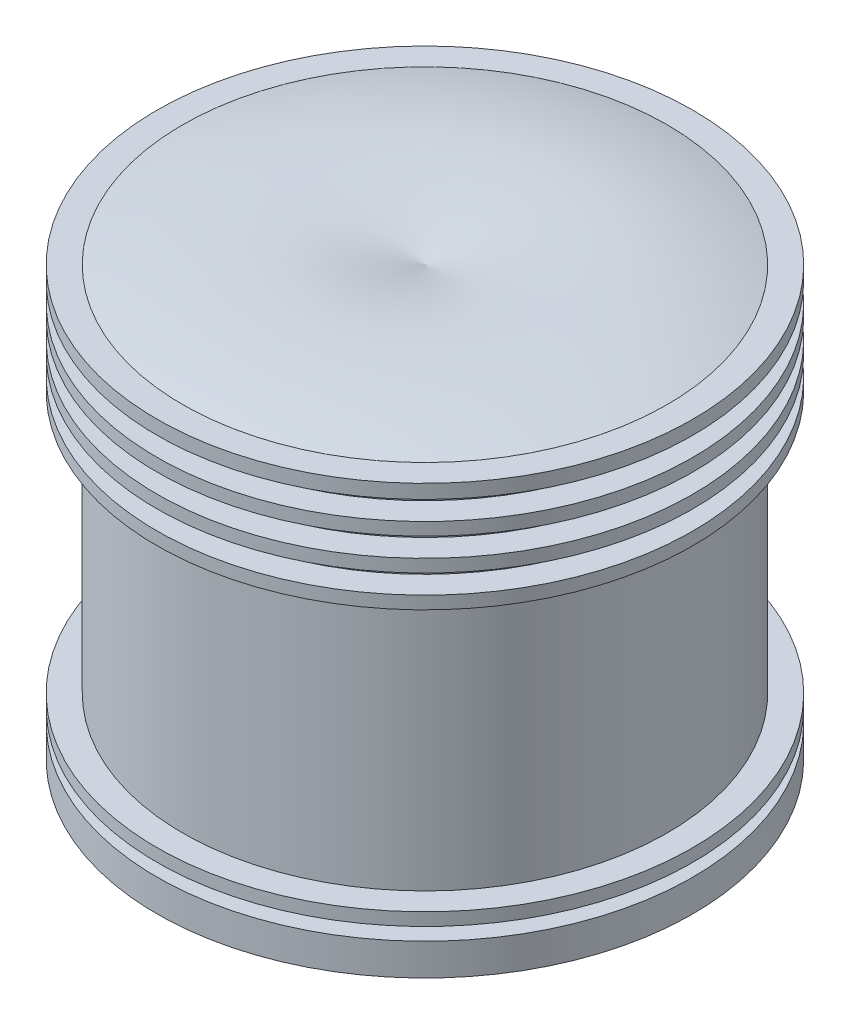
ISO-10303-21;
HEADER;
FILE_DESCRIPTION(('STEP AP214'),'2;1');
FILE_NAME('part.step','',(''),(''),'','','');
FILE_SCHEMA(('AUTOMOTIVE_DESIGN { 1 0 10303 214 1 1 1 1 }'));
ENDSEC;
DATA;
#1=APPLICATION_CONTEXT('core data for automotive mechanical design processes');
#2=APPLICATION_PROTOCOL_DEFINITION('international standard','automotive_design',2000,#1);
#3=PRODUCT_CONTEXT('',#1,'mechanical');
#4=PRODUCT('Part','Part','',(#3));
#5=PRODUCT_RELATED_PRODUCT_CATEGORY('part','',(#4));
#6=PRODUCT_DEFINITION_FORMATION('','',#4);
#7=PRODUCT_DEFINITION_CONTEXT('part definition',#1,'design');
#8=PRODUCT_DEFINITION('design','',#6,#7);
#9=PRODUCT_DEFINITION_SHAPE('','',#8);
#10=(LENGTH_UNIT() NAMED_UNIT(*) SI_UNIT(.MILLI.,.METRE.));
#11=(NAMED_UNIT(*) PLANE_ANGLE_UNIT() SI_UNIT($,.RADIAN.));
#12=(NAMED_UNIT(*) SI_UNIT($,.STERADIAN.) SOLID_ANGLE_UNIT());
#13=UNCERTAINTY_MEASURE_WITH_UNIT(LENGTH_MEASURE(1.E-05),#10,'distance_accuracy_value','');
#14=(GEOMETRIC_REPRESENTATION_CONTEXT(3) GLOBAL_UNCERTAINTY_ASSIGNED_CONTEXT((#13)) GLOBAL_UNIT_ASSIGNED_CONTEXT((#10,
#11,#12)) REPRESENTATION_CONTEXT('',''));
#15=CARTESIAN_POINT('',(0.,0.,0.));
#16=DIRECTION('',(0.,0.,1.));
#17=DIRECTION('',(1.,0.,0.));
#18=AXIS2_PLACEMENT_3D('',#15,#16,#17);
#19=CARTESIAN_POINT('',(0.,0.,0.));
#20=DIRECTION('',(0.,-1.,0.));
#21=DIRECTION('',(0.,0.,-1.));
#22=AXIS2_PLACEMENT_3D('',#19,#20,#21);
#23=CYLINDRICAL_SURFACE('',#22,42.);
#24=CARTESIAN_POINT('',(0.,9.,0.));
#25=DIRECTION('',(0.,-1.,0.));
#26=DIRECTION('',(0.,0.,-1.));
#27=AXIS2_PLACEMENT_3D('',#24,#25,#26);
#28=CIRCLE('',#27,42.);
#29=CARTESIAN_POINT('',(0.,9.,-42.));
#30=VERTEX_POINT('',#29);
#31=EDGE_CURVE('E171',#30,#30,#28,.T.);
#32=ORIENTED_EDGE('',*,*,#31,.T.);
#33=EDGE_LOOP('',(#32));
#34=FACE_BOUND('',#33,.T.);
#35=CARTESIAN_POINT('',(0.,7.,0.));
#36=DIRECTION('',(0.,-1.,0.));
#37=DIRECTION('',(0.,0.,-1.));
#38=AXIS2_PLACEMENT_3D('',#35,#36,#37);
#39=CIRCLE('',#38,42.);
#40=CARTESIAN_POINT('',(0.,7.,-42.));
#41=VERTEX_POINT('',#40);
#42=EDGE_CURVE('E11',#41,#41,#39,.T.);
#43=ORIENTED_EDGE('',*,*,#42,.F.);
#44=EDGE_LOOP('',(#43));
#45=FACE_BOUND('',#44,.T.);
#46=ADVANCED_FACE('F39',(#34,#45),#23,.T.);
#47=CARTESIAN_POINT('',(42.,7.,0.));
#48=DIRECTION('',(0.,-1.,0.));
#49=DIRECTION('',(0.,0.,-1.));
#50=AXIS2_PLACEMENT_3D('',#47,#48,#49);
#51=PLANE('',#50);
#52=ORIENTED_EDGE('',*,*,#42,.T.);
#53=EDGE_LOOP('',(#52));
#54=FACE_BOUND('',#53,.T.);
#55=CARTESIAN_POINT('',(0.,7.,0.));
#56=DIRECTION('',(0.,-1.,0.));
#57=DIRECTION('',(0.,0.,-1.));
#58=AXIS2_PLACEMENT_3D('',#55,#56,#57);
#59=CIRCLE('',#58,38.);
#60=CARTESIAN_POINT('',(0.,7.,-38.));
#61=VERTEX_POINT('',#60);
#62=EDGE_CURVE('E44',#61,#61,#59,.T.);
#63=ORIENTED_EDGE('',*,*,#62,.F.);
#64=EDGE_LOOP('',(#63));
#65=FACE_BOUND('',#64,.T.);
#66=ADVANCED_FACE('F80',(#54,#65),#51,.T.);
#67=CARTESIAN_POINT('',(0.,0.,0.));
#68=DIRECTION('',(0.,-1.,0.));
#69=DIRECTION('',(0.,0.,-1.));
#70=AXIS2_PLACEMENT_3D('',#67,#68,#69);
#71=CYLINDRICAL_SURFACE('',#70,38.);
#72=ORIENTED_EDGE('',*,*,#62,.T.);
#73=EDGE_LOOP('',(#72));
#74=FACE_BOUND('',#73,.T.);
#75=CARTESIAN_POINT('',(0.,5.,0.));
#76=DIRECTION('',(0.,-1.,0.));
#77=DIRECTION('',(0.,0.,-1.));
#78=AXIS2_PLACEMENT_3D('',#75,#76,#77);
#79=CIRCLE('',#78,38.);
#80=CARTESIAN_POINT('',(0.,5.,-38.));
#81=VERTEX_POINT('',#80);
#82=EDGE_CURVE('E73',#81,#81,#79,.T.);
#83=ORIENTED_EDGE('',*,*,#82,.F.);
#84=EDGE_LOOP('',(#83));
#85=FACE_BOUND('',#84,.T.);
#86=ADVANCED_FACE('F78',(#74,#85),#71,.T.);
#87=CARTESIAN_POINT('',(42.,5.,0.));
#88=DIRECTION('',(0.,1.,0.));
#89=DIRECTION('',(0.,0.,1.));
#90=AXIS2_PLACEMENT_3D('',#87,#88,#89);
#91=PLANE('',#90);
#92=ORIENTED_EDGE('',*,*,#82,.T.);
#93=EDGE_LOOP('',(#92));
#94=FACE_BOUND('',#93,.T.);
#95=CARTESIAN_POINT('',(0.,5.,0.));
#96=DIRECTION('',(0.,-1.,0.));
#97=DIRECTION('',(0.,0.,-1.));
#98=AXIS2_PLACEMENT_3D('',#95,#96,#97);
#99=CIRCLE('',#98,42.);
#100=CARTESIAN_POINT('',(0.,5.,-42.));
#101=VERTEX_POINT('',#100);
#102=EDGE_CURVE('E65',#101,#101,#99,.T.);
#103=ORIENTED_EDGE('',*,*,#102,.F.);
#104=EDGE_LOOP('',(#103));
#105=FACE_BOUND('',#104,.T.);
#106=ADVANCED_FACE('F86',(#94,#105),#91,.T.);
#107=CARTESIAN_POINT('',(0.,0.,0.));
#108=DIRECTION('',(0.,-1.,0.));
#109=DIRECTION('',(0.,0.,-1.));
#110=AXIS2_PLACEMENT_3D('',#107,#108,#109);
#111=CYLINDRICAL_SURFACE('',#110,42.);
#112=ORIENTED_EDGE('',*,*,#102,.T.);
#113=EDGE_LOOP('',(#112));
#114=FACE_BOUND('',#113,.T.);
#115=CARTESIAN_POINT('',(0.,0.,0.));
#116=DIRECTION('',(0.,-1.,0.));
#117=DIRECTION('',(0.,0.,-1.));
#118=AXIS2_PLACEMENT_3D('',#115,#116,#117);
#119=CIRCLE('',#118,42.);
#120=CARTESIAN_POINT('',(0.,0.,-42.));
#121=VERTEX_POINT('',#120);
#122=EDGE_CURVE('E59',#121,#121,#119,.T.);
#123=ORIENTED_EDGE('',*,*,#122,.F.);
#124=EDGE_LOOP('',(#123));
#125=FACE_BOUND('',#124,.T.);
#126=ADVANCED_FACE('F95',(#114,#125),#111,.T.);
#127=CARTESIAN_POINT('',(0.,0.,0.));
#128=DIRECTION('',(0.,-1.,0.));
#129=DIRECTION('',(0.,0.,-1.));
#130=AXIS2_PLACEMENT_3D('',#127,#128,#129);
#131=PLANE('',#130);
#132=ORIENTED_EDGE('',*,*,#122,.T.);
#133=EDGE_LOOP('',(#132));
#134=FACE_BOUND('',#133,.T.);
#135=ADVANCED_FACE('F55',(#134),#131,.T.);
#136=CARTESIAN_POINT('',(0.,-0.407583241532755,-19.));
#137=DIRECTION('',(-1.,0.,0.));
#138=DIRECTION('',(0.,0.,-1.));
#139=AXIS2_PLACEMENT_3D('',#136,#137,#138);
#140=CIRCLE('',#139,70.2095288278656);
#141=TRIMMED_CURVE('',#140,(PARAMETER_VALUE(-1.84483181190516)),
(PARAMETER_VALUE(1.84483181190516)),.T.,.PARAMETER.);
#142=CARTESIAN_POINT('',(0.,-0.407583241532755,0.));
#143=DIRECTION('',(0.,-1.,0.));
#144=AXIS1_PLACEMENT('',#142,#143);
#145=SURFACE_OF_REVOLUTION('',#141,#144);
#146=CARTESIAN_POINT('',(0.,67.1821936350844,0.));
#147=VERTEX_POINT('',#146);
#148=VERTEX_LOOP('',#147);
#149=FACE_BOUND('',#148,.T.);
#150=CARTESIAN_POINT('',(0.,67.1821936350844,0.));
#151=DIRECTION('',(0.,-1.,0.));
#152=DIRECTION('',(0.,0.,-1.));
#153=AXIS2_PLACEMENT_3D('',#150,#151,#152);
#154=CIRCLE('',#153,38.);
#155=CARTESIAN_POINT('',(0.,67.1821936350844,-38.));
#156=VERTEX_POINT('',#155);
#157=EDGE_CURVE('E57',#156,#156,#154,.T.);
#158=ORIENTED_EDGE('',*,*,#157,.F.);
#159=EDGE_LOOP('',(#158));
#160=FACE_BOUND('',#159,.T.);
#161=ADVANCED_FACE('F48',(#149,#160),#145,.T.);
#162=CARTESIAN_POINT('',(38.,67.1821936350844,0.));
#163=DIRECTION('',(0.,1.,0.));
#164=DIRECTION('',(0.,0.,1.));
#165=AXIS2_PLACEMENT_3D('',#162,#163,#164);
#166=PLANE('',#165);
#167=ORIENTED_EDGE('',*,*,#157,.T.);
#168=EDGE_LOOP('',(#167));
#169=FACE_BOUND('',#168,.T.);
#170=CARTESIAN_POINT('',(0.,67.1821936350844,0.));
#171=DIRECTION('',(0.,-1.,0.));
#172=DIRECTION('',(0.,0.,-1.));
#173=AXIS2_PLACEMENT_3D('',#170,#171,#172);
#174=CIRCLE('',#173,42.);
#175=CARTESIAN_POINT('',(0.,67.1821936350844,-42.));
#176=VERTEX_POINT('',#175);
#177=EDGE_CURVE('E56',#176,#176,#174,.T.);
#178=ORIENTED_EDGE('',*,*,#177,.F.);
#179=EDGE_LOOP('',(#178));
#180=FACE_BOUND('',#179,.T.);
#181=ADVANCED_FACE('F51',(#169,#180),#166,.T.);
#182=CARTESIAN_POINT('',(0.,0.,0.));
#183=DIRECTION('',(0.,-1.,0.));
#184=DIRECTION('',(0.,0.,-1.));
#185=AXIS2_PLACEMENT_3D('',#182,#183,#184);
#186=CYLINDRICAL_SURFACE('',#185,42.);
#187=ORIENTED_EDGE('',*,*,#177,.T.);
#188=EDGE_LOOP('',(#187));
#189=FACE_BOUND('',#188,.T.);
#190=CARTESIAN_POINT('',(0.,65.,0.));
#191=DIRECTION('',(0.,-1.,0.));
#192=DIRECTION('',(0.,0.,-1.));
#193=AXIS2_PLACEMENT_3D('',#190,#191,#192);
#194=CIRCLE('',#193,42.);
#195=CARTESIAN_POINT('',(0.,65.,-42.));
#196=VERTEX_POINT('',#195);
#197=EDGE_CURVE('E64',#196,#196,#194,.T.);
#198=ORIENTED_EDGE('',*,*,#197,.F.);
#199=EDGE_LOOP('',(#198));
#200=FACE_BOUND('',#199,.T.);
#201=ADVANCED_FACE('F105',(#189,#200),#186,.T.);
#202=CARTESIAN_POINT('',(42.,65.,0.));
#203=DIRECTION('',(0.,-1.,0.));
#204=DIRECTION('',(0.,0.,-1.));
#205=AXIS2_PLACEMENT_3D('',#202,#203,#204);
#206=PLANE('',#205);
#207=ORIENTED_EDGE('',*,*,#197,.T.);
#208=EDGE_LOOP('',(#207));
#209=FACE_BOUND('',#208,.T.);
#210=CARTESIAN_POINT('',(0.,65.,0.));
#211=DIRECTION('',(0.,-1.,0.));
#212=DIRECTION('',(0.,0.,-1.));
#213=AXIS2_PLACEMENT_3D('',#210,#211,#212);
#214=CIRCLE('',#213,38.);
#215=CARTESIAN_POINT('',(0.,65.,-38.));
#216=VERTEX_POINT('',#215);
#217=EDGE_CURVE('E211',#216,#216,#214,.T.);
#218=ORIENTED_EDGE('',*,*,#217,.F.);
#219=EDGE_LOOP('',(#218));
#220=FACE_BOUND('',#219,.T.);
#221=ADVANCED_FACE('F103',(#209,#220),#206,.T.);
#222=CARTESIAN_POINT('',(0.,0.,0.));
#223=DIRECTION('',(0.,-1.,0.));
#224=DIRECTION('',(0.,0.,-1.));
#225=AXIS2_PLACEMENT_3D('',#222,#223,#224);
#226=CYLINDRICAL_SURFACE('',#225,38.);
#227=ORIENTED_EDGE('',*,*,#217,.T.);
#228=EDGE_LOOP('',(#227));
#229=FACE_BOUND('',#228,.T.);
#230=CARTESIAN_POINT('',(0.,62.,0.));
#231=DIRECTION('',(0.,-1.,0.));
#232=DIRECTION('',(0.,0.,-1.));
#233=AXIS2_PLACEMENT_3D('',#230,#231,#232);
#234=CIRCLE('',#233,38.);
#235=CARTESIAN_POINT('',(0.,62.,-38.));
#236=VERTEX_POINT('',#235);
#237=EDGE_CURVE('E209',#236,#236,#234,.T.);
#238=ORIENTED_EDGE('',*,*,#237,.F.);
#239=EDGE_LOOP('',(#238));
#240=FACE_BOUND('',#239,.T.);
#241=ADVANCED_FACE('F107',(#229,#240),#226,.T.);
#242=CARTESIAN_POINT('',(38.,62.,0.));
#243=DIRECTION('',(0.,1.,0.));
#244=DIRECTION('',(0.,0.,1.));
#245=AXIS2_PLACEMENT_3D('',#242,#243,#244);
#246=PLANE('',#245);
#247=ORIENTED_EDGE('',*,*,#237,.T.);
#248=EDGE_LOOP('',(#247));
#249=FACE_BOUND('',#248,.T.);
#250=CARTESIAN_POINT('',(0.,62.,0.));
#251=DIRECTION('',(0.,-1.,0.));
#252=DIRECTION('',(0.,0.,-1.));
#253=AXIS2_PLACEMENT_3D('',#250,#251,#252);
#254=CIRCLE('',#253,42.);
#255=CARTESIAN_POINT('',(0.,62.,-42.));
#256=VERTEX_POINT('',#255);
#257=EDGE_CURVE('E210',#256,#256,#254,.T.);
#258=ORIENTED_EDGE('',*,*,#257,.F.);
#259=EDGE_LOOP('',(#258));
#260=FACE_BOUND('',#259,.T.);
#261=ADVANCED_FACE('F111',(#249,#260),#246,.T.);
#262=CARTESIAN_POINT('',(0.,0.,0.));
#263=DIRECTION('',(0.,-1.,0.));
#264=DIRECTION('',(0.,0.,-1.));
#265=AXIS2_PLACEMENT_3D('',#262,#263,#264);
#266=CYLINDRICAL_SURFACE('',#265,42.);
#267=ORIENTED_EDGE('',*,*,#257,.T.);
#268=EDGE_LOOP('',(#267));
#269=FACE_BOUND('',#268,.T.);
#270=CARTESIAN_POINT('',(0.,60.,0.));
#271=DIRECTION('',(0.,-1.,0.));
#272=DIRECTION('',(0.,0.,-1.));
#273=AXIS2_PLACEMENT_3D('',#270,#271,#272);
#274=CIRCLE('',#273,42.);
#275=CARTESIAN_POINT('',(0.,60.,-42.));
#276=VERTEX_POINT('',#275);
#277=EDGE_CURVE('E204',#276,#276,#274,.T.);
#278=ORIENTED_EDGE('',*,*,#277,.F.);
#279=EDGE_LOOP('',(#278));
#280=FACE_BOUND('',#279,.T.);
#281=ADVANCED_FACE('F120',(#269,#280),#266,.T.);
#282=CARTESIAN_POINT('',(42.,60.,0.));
#283=DIRECTION('',(0.,-1.,0.));
#284=DIRECTION('',(0.,0.,-1.));
#285=AXIS2_PLACEMENT_3D('',#282,#283,#284);
#286=PLANE('',#285);
#287=ORIENTED_EDGE('',*,*,#277,.T.);
#288=EDGE_LOOP('',(#287));
#289=FACE_BOUND('',#288,.T.);
#290=CARTESIAN_POINT('',(0.,60.,0.));
#291=DIRECTION('',(0.,-1.,0.));
#292=DIRECTION('',(0.,0.,-1.));
#293=AXIS2_PLACEMENT_3D('',#290,#291,#292);
#294=CIRCLE('',#293,38.);
#295=CARTESIAN_POINT('',(0.,60.,-38.));
#296=VERTEX_POINT('',#295);
#297=EDGE_CURVE('E202',#296,#296,#294,.T.);
#298=ORIENTED_EDGE('',*,*,#297,.F.);
#299=EDGE_LOOP('',(#298));
#300=FACE_BOUND('',#299,.T.);
#301=ADVANCED_FACE('F123',(#289,#300),#286,.T.);
#302=CARTESIAN_POINT('',(0.,0.,0.));
#303=DIRECTION('',(0.,-1.,0.));
#304=DIRECTION('',(0.,0.,-1.));
#305=AXIS2_PLACEMENT_3D('',#302,#303,#304);
#306=CYLINDRICAL_SURFACE('',#305,38.);
#307=ORIENTED_EDGE('',*,*,#297,.T.);
#308=EDGE_LOOP('',(#307));
#309=FACE_BOUND('',#308,.T.);
#310=CARTESIAN_POINT('',(0.,57.,0.));
#311=DIRECTION('',(0.,-1.,0.));
#312=DIRECTION('',(0.,0.,-1.));
#313=AXIS2_PLACEMENT_3D('',#310,#311,#312);
#314=CIRCLE('',#313,38.);
#315=CARTESIAN_POINT('',(0.,57.,-38.));
#316=VERTEX_POINT('',#315);
#317=EDGE_CURVE('E196',#316,#316,#314,.T.);
#318=ORIENTED_EDGE('',*,*,#317,.F.);
#319=EDGE_LOOP('',(#318));
#320=FACE_BOUND('',#319,.T.);
#321=ADVANCED_FACE('F124',(#309,#320),#306,.T.);
#322=CARTESIAN_POINT('',(38.,57.,0.));
#323=DIRECTION('',(0.,1.,0.));
#324=DIRECTION('',(0.,0.,1.));
#325=AXIS2_PLACEMENT_3D('',#322,#323,#324);
#326=PLANE('',#325);
#327=ORIENTED_EDGE('',*,*,#317,.T.);
#328=EDGE_LOOP('',(#327));
#329=FACE_BOUND('',#328,.T.);
#330=CARTESIAN_POINT('',(0.,57.,0.));
#331=DIRECTION('',(0.,-1.,0.));
#332=DIRECTION('',(0.,0.,-1.));
#333=AXIS2_PLACEMENT_3D('',#330,#331,#332);
#334=CIRCLE('',#333,42.);
#335=CARTESIAN_POINT('',(0.,57.,-42.));
#336=VERTEX_POINT('',#335);
#337=EDGE_CURVE('E193',#336,#336,#334,.T.);
#338=ORIENTED_EDGE('',*,*,#337,.F.);
#339=EDGE_LOOP('',(#338));
#340=FACE_BOUND('',#339,.T.);
#341=ADVANCED_FACE('F129',(#329,#340),#326,.T.);
#342=CARTESIAN_POINT('',(0.,0.,0.));
#343=DIRECTION('',(0.,-1.,0.));
#344=DIRECTION('',(0.,0.,-1.));
#345=AXIS2_PLACEMENT_3D('',#342,#343,#344);
#346=CYLINDRICAL_SURFACE('',#345,42.);
#347=ORIENTED_EDGE('',*,*,#337,.T.);
#348=EDGE_LOOP('',(#347));
#349=FACE_BOUND('',#348,.T.);
#350=CARTESIAN_POINT('',(0.,55.,0.));
#351=DIRECTION('',(0.,-1.,0.));
#352=DIRECTION('',(0.,0.,-1.));
#353=AXIS2_PLACEMENT_3D('',#350,#351,#352);
#354=CIRCLE('',#353,42.);
#355=CARTESIAN_POINT('',(0.,55.,-42.));
#356=VERTEX_POINT('',#355);
#357=EDGE_CURVE('E195',#356,#356,#354,.T.);
#358=ORIENTED_EDGE('',*,*,#357,.F.);
#359=EDGE_LOOP('',(#358));
#360=FACE_BOUND('',#359,.T.);
#361=ADVANCED_FACE('F133',(#349,#360),#346,.T.);
#362=CARTESIAN_POINT('',(42.,55.,0.));
#363=DIRECTION('',(0.,-1.,0.));
#364=DIRECTION('',(0.,0.,-1.));
#365=AXIS2_PLACEMENT_3D('',#362,#363,#364);
#366=PLANE('',#365);
#367=ORIENTED_EDGE('',*,*,#357,.T.);
#368=EDGE_LOOP('',(#367));
#369=FACE_BOUND('',#368,.T.);
#370=CARTESIAN_POINT('',(0.,55.,0.));
#371=DIRECTION('',(0.,-1.,0.));
#372=DIRECTION('',(0.,0.,-1.));
#373=AXIS2_PLACEMENT_3D('',#370,#371,#372);
#374=CIRCLE('',#373,38.);
#375=CARTESIAN_POINT('',(0.,55.,-38.));
#376=VERTEX_POINT('',#375);
#377=EDGE_CURVE('E188',#376,#376,#374,.T.);
#378=ORIENTED_EDGE('',*,*,#377,.F.);
#379=EDGE_LOOP('',(#378));
#380=FACE_BOUND('',#379,.T.);
#381=ADVANCED_FACE('F140',(#369,#380),#366,.T.);
#382=CARTESIAN_POINT('',(0.,0.,0.));
#383=DIRECTION('',(0.,-1.,0.));
#384=DIRECTION('',(0.,0.,-1.));
#385=AXIS2_PLACEMENT_3D('',#382,#383,#384);
#386=CYLINDRICAL_SURFACE('',#385,38.);
#387=ORIENTED_EDGE('',*,*,#377,.T.);
#388=EDGE_LOOP('',(#387));
#389=FACE_BOUND('',#388,.T.);
#390=CARTESIAN_POINT('',(0.,52.,0.));
#391=DIRECTION('',(0.,-1.,0.));
#392=DIRECTION('',(0.,0.,-1.));
#393=AXIS2_PLACEMENT_3D('',#390,#391,#392);
#394=CIRCLE('',#393,38.);
#395=CARTESIAN_POINT('',(0.,52.,-38.));
#396=VERTEX_POINT('',#395);
#397=EDGE_CURVE('E186',#396,#396,#394,.T.);
#398=ORIENTED_EDGE('',*,*,#397,.F.);
#399=EDGE_LOOP('',(#398));
#400=FACE_BOUND('',#399,.T.);
#401=ADVANCED_FACE('F141',(#389,#400),#386,.T.);
#402=CARTESIAN_POINT('',(38.,52.,0.));
#403=DIRECTION('',(0.,1.,0.));
#404=DIRECTION('',(0.,0.,1.));
#405=AXIS2_PLACEMENT_3D('',#402,#403,#404);
#406=PLANE('',#405);
#407=ORIENTED_EDGE('',*,*,#397,.T.);
#408=EDGE_LOOP('',(#407));
#409=FACE_BOUND('',#408,.T.);
#410=CARTESIAN_POINT('',(0.,52.,0.));
#411=DIRECTION('',(0.,-1.,0.));
#412=DIRECTION('',(0.,0.,-1.));
#413=AXIS2_PLACEMENT_3D('',#410,#411,#412);
#414=CIRCLE('',#413,42.);
#415=CARTESIAN_POINT('',(0.,52.,-42.));
#416=VERTEX_POINT('',#415);
#417=EDGE_CURVE('E183',#416,#416,#414,.T.);
#418=ORIENTED_EDGE('',*,*,#417,.F.);
#419=EDGE_LOOP('',(#418));
#420=FACE_BOUND('',#419,.T.);
#421=ADVANCED_FACE('F144',(#409,#420),#406,.T.);
#422=CARTESIAN_POINT('',(0.,0.,0.));
#423=DIRECTION('',(0.,-1.,0.));
#424=DIRECTION('',(0.,0.,-1.));
#425=AXIS2_PLACEMENT_3D('',#422,#423,#424);
#426=CYLINDRICAL_SURFACE('',#425,42.);
#427=ORIENTED_EDGE('',*,*,#417,.T.);
#428=EDGE_LOOP('',(#427));
#429=FACE_BOUND('',#428,.T.);
#430=CARTESIAN_POINT('',(0.,50.,0.));
#431=DIRECTION('',(0.,-1.,0.));
#432=DIRECTION('',(0.,0.,-1.));
#433=AXIS2_PLACEMENT_3D('',#430,#431,#432);
#434=CIRCLE('',#433,42.);
#435=CARTESIAN_POINT('',(0.,50.,-42.));
#436=VERTEX_POINT('',#435);
#437=EDGE_CURVE('E179',#436,#436,#434,.T.);
#438=ORIENTED_EDGE('',*,*,#437,.F.);
#439=EDGE_LOOP('',(#438));
#440=FACE_BOUND('',#439,.T.);
#441=ADVANCED_FACE('F146',(#429,#440),#426,.T.);
#442=CARTESIAN_POINT('',(42.,50.,0.));
#443=DIRECTION('',(0.,-1.,0.));
#444=DIRECTION('',(0.,0.,-1.));
#445=AXIS2_PLACEMENT_3D('',#442,#443,#444);
#446=PLANE('',#445);
#447=ORIENTED_EDGE('',*,*,#437,.T.);
#448=EDGE_LOOP('',(#447));
#449=FACE_BOUND('',#448,.T.);
#450=CARTESIAN_POINT('',(0.,50.,0.));
#451=DIRECTION('',(0.,-1.,0.));
#452=DIRECTION('',(0.,0.,-1.));
#453=AXIS2_PLACEMENT_3D('',#450,#451,#452);
#454=CIRCLE('',#453,38.);
#455=CARTESIAN_POINT('',(0.,50.,-38.));
#456=VERTEX_POINT('',#455);
#457=EDGE_CURVE('E172',#456,#456,#454,.T.);
#458=ORIENTED_EDGE('',*,*,#457,.F.);
#459=EDGE_LOOP('',(#458));
#460=FACE_BOUND('',#459,.T.);
#461=ADVANCED_FACE('F151',(#449,#460),#446,.T.);
#462=CARTESIAN_POINT('',(0.,0.,0.));
#463=DIRECTION('',(0.,-1.,0.));
#464=DIRECTION('',(0.,0.,-1.));
#465=AXIS2_PLACEMENT_3D('',#462,#463,#464);
#466=CYLINDRICAL_SURFACE('',#465,38.);
#467=ORIENTED_EDGE('',*,*,#457,.T.);
#468=EDGE_LOOP('',(#467));
#469=FACE_BOUND('',#468,.T.);
#470=CARTESIAN_POINT('',(0.,9.,0.));
#471=DIRECTION('',(0.,-1.,0.));
#472=DIRECTION('',(0.,0.,-1.));
#473=AXIS2_PLACEMENT_3D('',#470,#471,#472);
#474=CIRCLE('',#473,38.);
#475=CARTESIAN_POINT('',(0.,9.,-38.));
#476=VERTEX_POINT('',#475);
#477=EDGE_CURVE('E169',#476,#476,#474,.T.);
#478=ORIENTED_EDGE('',*,*,#477,.F.);
#479=EDGE_LOOP('',(#478));
#480=FACE_BOUND('',#479,.T.);
#481=ADVANCED_FACE('F160',(#469,#480),#466,.T.);
#482=CARTESIAN_POINT('',(42.,9.,0.));
#483=DIRECTION('',(0.,1.,0.));
#484=DIRECTION('',(0.,0.,1.));
#485=AXIS2_PLACEMENT_3D('',#482,#483,#484);
#486=PLANE('',#485);
#487=ORIENTED_EDGE('',*,*,#477,.T.);
#488=EDGE_LOOP('',(#487));
#489=FACE_BOUND('',#488,.T.);
#490=ORIENTED_EDGE('',*,*,#31,.F.);
#491=EDGE_LOOP('',(#490));
#492=FACE_BOUND('',#491,.T.);
#493=ADVANCED_FACE('F163',(#489,#492),#486,.T.);
#494=CLOSED_SHELL('',(#46,#66,#86,#106,#126,#135,#161,#181,#201,#221,#241,#261,#281,#301,#321,
#341,#361,#381,#401,#421,#441,#461,#481,#493));
#495=MANIFOLD_SOLID_BREP('B2',#494);
#496=ADVANCED_BREP_SHAPE_REPRESENTATION('',(#18,#495),#14);
#497=SHAPE_DEFINITION_REPRESENTATION(#9,#496);
ENDSEC;
END-ISO-10303-21;
